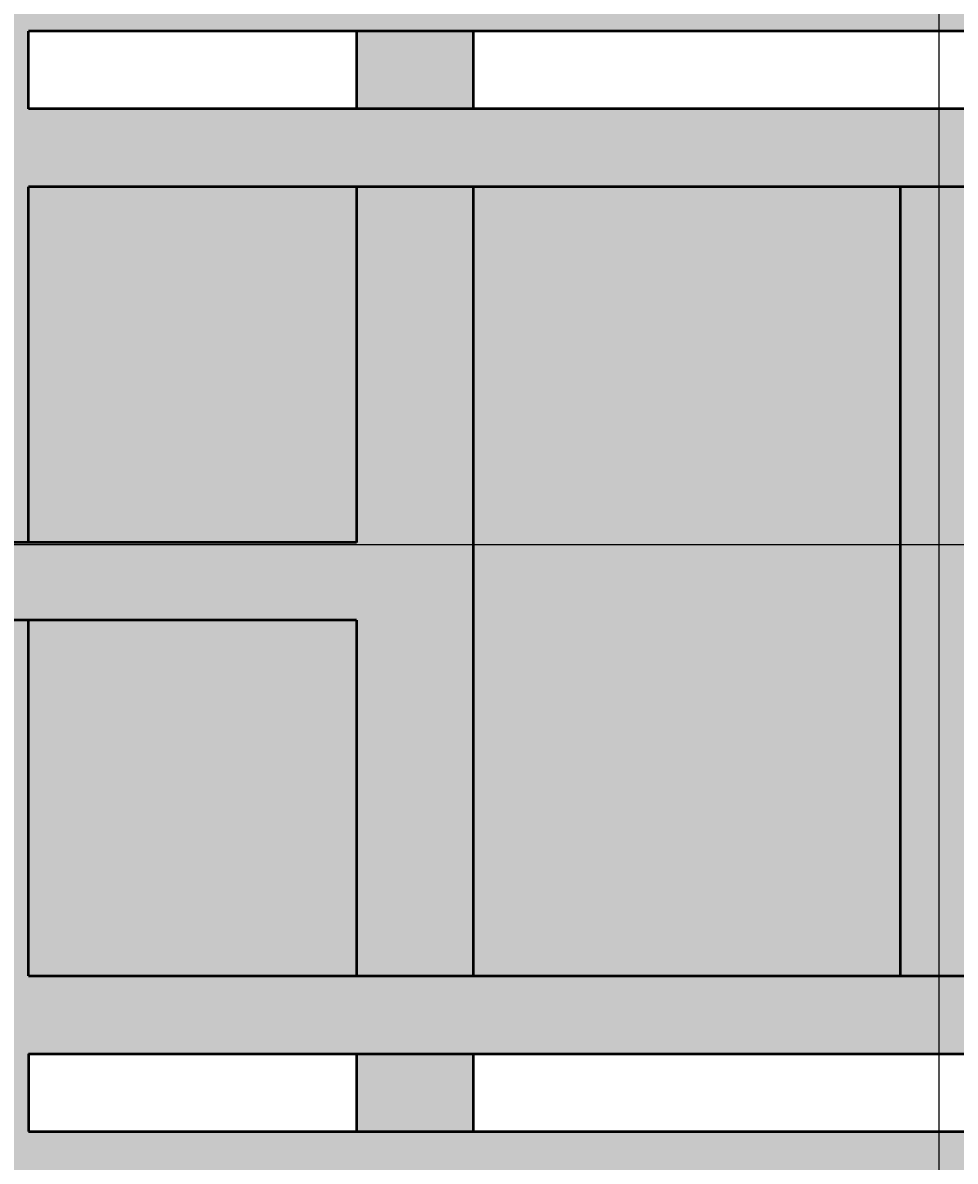
# Model space of a CAD drawing. Units: inches. Extents: x -12 to 334, y -10 to 186.
# Tile 17 of 77: x 64 to 88, y 65 to 94. Entities that reach past the tile are written whole.
import ezdxf

# ---------------------------------------------------------------- set-up
doc = ezdxf.new("R2010")
doc.units = ezdxf.units.IN
doc.header["$MEASUREMENT"] = 0
for name, color, linetype, lineweight in [('M-DIMS', 2, 'Continuous', 18), ('M-EQPM', 7, 'Continuous', 50), ('M-EQPM-PATT', 8, 'Continuous', 18)]:
    doc.layers.add(name, color=color, linetype=linetype, lineweight=lineweight)
doc.styles.get("Standard").update_dxf_attribs({"font": 'arial.ttf'})
doc.dimstyles.get("Standard").update_dxf_attribs({"dimtxt": 0.18, "dimasz": 0.18, "dimexe": 0.18, "dimexo": 0.0625, "dimgap": 0.09, "dimtad": 0, "dimtih": 1, "dimtoh": 1, "dimdec": 4, "dimzin": 0, "dimdsep": 46, "dimtxsty": 'Standard', "dimcen": 0.09, "dimadec": 0, "dimazin": 0, "dimtfac": 1, "dimtdec": 4, "dimtofl": 0, "dimtmove": 0, "dimatfit": 3, "dimfxl": 1, "dimtolj": 1, "dimtzin": 0, "dimarcsym": 0})

# ---------------------------------------------------------------- blocks, each defined once
blk = doc.blocks.new('*D1')
at = {"layer": 'Defpoints', "color": 0, "transparency": 16777216}
for p in [(281.426, 91.899), (3.376, 80.692), (281.426, 14.304)]:
    blk.add_point(p, dxfattribs=at)
at = {"layer": 'M-DIMS', "color": 0, "lineweight": -2, "transparency": 16777216}
for p, q in [((281.426, 91.836), (281.426, 14.124)), ((3.376, 80.629), (3.376, 14.124)), ((3.556, 14.304), (141.935, 14.304)), ((281.246, 14.304), (142.867, 14.304))]:
    blk.add_line(p, q, dxfattribs=at)
at = {"layer": 'M-DIMS', "color": 0, "transparency": 16777216}
for points in [[(3.556, 14.334), (3.556, 14.274), (3.376, 14.304)], [(281.246, 14.334), (281.246, 14.274), (281.426, 14.304)]]:
    blk.add_solid(points, dxfattribs=at)
at = {"layer": 'M-DIMS', "color": 0, "transparency": 16777216, "insert": (142.401, 14.304), "char_height": 0.18, "attachment_point": 5}
blk.add_mtext('\\A1;278.05', dxfattribs=at)
blk = doc.blocks.new('*D26')
at = {"layer": 'Defpoints', "color": 0, "transparency": 16777216}
for p in [(87.888, 169.385), (87.888, 56.321), (58.1, 33.675)]:
    blk.add_point(p, dxfattribs=at)
at = {"layer": 'M-DIMS', "color": 0, "lineweight": -2, "transparency": 16777216}
for p, q in [((58.1, 33.738), (58.1, 169.565)), ((87.888, 56.383), (87.888, 169.565)), ((58.28, 169.385), (72.599, 169.385)), ((87.708, 169.385), (73.389, 169.385))]:
    blk.add_line(p, q, dxfattribs=at)
at = {"layer": 'M-DIMS', "color": 0, "transparency": 16777216}
for points in [[(58.28, 169.415), (58.28, 169.355), (58.1, 169.385)], [(87.708, 169.415), (87.708, 169.355), (87.888, 169.385)]]:
    blk.add_solid(points, dxfattribs=at)
at = {"layer": 'M-DIMS', "color": 0, "transparency": 16777216, "insert": (72.994, 169.385), "char_height": 0.18, "attachment_point": 5}
blk.add_mtext('\\A1;29.79', dxfattribs=at)
blk = doc.blocks.new('*D35')
at = {"layer": 'Defpoints', "color": 0, "transparency": 16777216}
for p in [(216.428, 98.108), (-11.174, 61.105), (216.428, 61.105)]:
    blk.add_point(p, dxfattribs=at)
at = {"layer": 'M-DIMS', "color": 0, "lineweight": -2, "transparency": 16777216}
for p, q in [((216.365, 98.108), (-11.354, 98.108)), ((-11.174, 97.928), (-11.174, 79.788)), ((-11.174, 61.285), (-11.174, 79.424)), ((216.365, 61.105), (-11.354, 61.105))]:
    blk.add_line(p, q, dxfattribs=at)
at = {"layer": 'M-DIMS', "color": 0, "transparency": 16777216}
for points in [[(-11.204, 97.928), (-11.144, 97.928), (-11.174, 98.108)], [(-11.204, 61.285), (-11.144, 61.285), (-11.174, 61.105)]]:
    blk.add_solid(points, dxfattribs=at)
at = {"layer": 'M-DIMS', "color": 0, "transparency": 16777216, "insert": (-11.174, 79.606), "char_height": 0.18, "attachment_point": 5}
blk.add_mtext('\\A1;37', dxfattribs=at)
blk = doc.blocks.new('*D39')
at = {"layer": 'Defpoints', "color": 0, "transparency": 16777216}
for p in [(279.726, 80.692), (-11.174, 45.854), (269.381, 45.854)]:
    blk.add_point(p, dxfattribs=at)
at = {"layer": 'M-DIMS', "color": 0, "lineweight": -2, "transparency": 16777216}
for p, q in [((279.664, 80.692), (-11.354, 80.692)), ((-11.174, 80.512), (-11.174, 63.455)), ((-11.174, 46.034), (-11.174, 63.091)), ((269.318, 45.854), (-11.354, 45.854))]:
    blk.add_line(p, q, dxfattribs=at)
at = {"layer": 'M-DIMS', "color": 0, "transparency": 16777216}
for points in [[(-11.204, 80.512), (-11.144, 80.512), (-11.174, 80.692)], [(-11.204, 46.034), (-11.144, 46.034), (-11.174, 45.854)]]:
    blk.add_solid(points, dxfattribs=at)
at = {"layer": 'M-DIMS', "color": 0, "transparency": 16777216, "insert": (-11.174, 63.273), "char_height": 0.18, "attachment_point": 5}
blk.add_mtext('\\A1;34.84', dxfattribs=at)

msp = doc.modelspace()

# ---------------------------------------------------------------- hatches: boundary and pattern name
at = {"layer": 'M-EQPM-PATT'}
h = msp.add_hatch(color=256, dxfattribs=at)
h.set_gradient(color1=(99, 100, 102), color2=(99, 100, 102), tint=1)
h.paths.add_polyline_path([(4.3766, 80.754, -0.4132606), (23.5807, 99.8958), (37.1002, 99.8958), (37.1002, 127.7078), (32.1002, 127.7078), (32.1002, 125.2078), (36.1002, 125.2078), (36.1002, 100.8958), (23.5807, 100.8958, 1), (23.5807, 60.4872), (36.1002, 60.4872), (36.1002, 36.1752), (32.1002, 36.1752), (32.1002, 33.6752), (37.1002, 33.6752), (37.1002, 61.4872), (23.5807, 61.4872, -0.384914), (4.4744, 78.754), (72.9244, 78.754), (72.9244, 69.6117), (75.9244, 69.6117), (75.9244, 89.8963), (72.9244, 89.8963), (72.9244, 80.754)])
h.paths.add_polyline_path([(54.1002, 125.2078), (58.1002, 125.2078), (58.1002, 127.7078), (53.1002, 127.7078), (53.1002, 99.8958), (64.5, 99.8958), (64.5, 109.0583), (63.5, 109.0583), (63.5, 100.8958), (54.1002, 100.8958)], flags=17)
h.paths.add_polyline_path([(53.1002, 33.6752), (58.1002, 33.6752), (58.1002, 36.1752), (54.1002, 36.1752), (54.1002, 60.4872), (64.2068, 60.4872), (64.2068, 49.4497), (87.8879, 49.4497), (87.8879, 55.3205), (104.8919, 55.3205), (104.8919, 30.8541), (99.8919, 30.8541), (99.8919, 28.8541), (105.8919, 28.8541), (105.8919, 56.3205), (87.8879, 56.3205), (87.8879, 63.6117), (86.8879, 63.6117), (86.8879, 50.4497), (65.0061, 50.4497), (65.0061, 63.6117), (64.5, 63.6117), (64.5, 61.4872), (53.1002, 61.4872)])
h.paths.add_polyline_path([(121.8919, 28.8541), (121.8919, 30.8541), (116.8919, 30.8541), (116.8919, 45.8541), (209.6965, 45.8541), (209.9204, 46.8541), (115.8919, 46.8541), (115.8919, 28.8541)])
h.paths.add_polyline_path([(221.5761, 32.8541), (216.5761, 32.8541), (216.5761, 30.8541), (222.5761, 30.8541), (222.5761, 46.8541), (209.9204, 46.8541), (209.6965, 45.8541), (221.5761, 45.8541)])
h.paths.add_polyline_path([(233.5761, 45.8541), (249.8485, 45.8541), (249.3759, 46.8541), (232.5761, 46.8541), (232.5761, 30.8541), (238.5761, 30.8541), (238.5761, 32.8541), (233.5761, 32.8541)])
h = msp.add_hatch(color=256, dxfattribs=at)
h.set_gradient(color1=(205, 32, 39), color2=(205, 32, 39), tint=1)
h.paths.add_polyline_path([(64.5, 80.754), (64.5, 89.8963), (226.6083, 89.8963, -1), (226.6083, 69.6117), (64.5, 69.6117), (64.5, 78.754), (4.4744, 78.754, 0.384914), (23.5807, 61.4872), (37.1002, 61.4872), (37.1002, 33.6752), (53.1002, 33.6752), (53.1002, 61.4872), (64.5, 61.4872), (64.5, 63.6117), (226.6083, 63.6117, 1), (226.6083, 95.8963), (64.5, 95.8963), (64.5, 99.8958), (53.1002, 99.8958), (53.1002, 127.7078), (37.1002, 127.7078), (37.1002, 99.8958), (23.5807, 99.8958, 0.4132606), (4.3766, 80.754)])
h.paths.add_polyline_path([(64.5, 91.8963), (64.5, 93.8963), (226.6083, 93.8963, -1), (226.6083, 65.6117), (64.5, 65.6117), (64.5, 67.6117), (226.6083, 67.6117, 1), (226.6083, 91.8963)], flags=16)
h = msp.add_hatch(color=256, dxfattribs=at)
h.set_gradient(color1=(205, 32, 39), color2=(205, 32, 39), tint=1)
h.paths.add_polyline_path([(72.9244, 95.8963), (72.9244, 109.0583), (64.5, 109.0583), (64.5, 95.8963)])
h.paths.add_polyline_path([(72.9244, 80.754), (72.9244, 89.8963), (64.5, 89.8963), (64.5, 80.754)])
h.paths.add_polyline_path([(72.9244, 69.6117), (72.9244, 78.754), (64.5, 78.754), (64.5, 69.6117)])
h.paths.add_polyline_path([(72.9244, 50.4497), (72.9244, 63.6117), (65.0061, 63.6117), (65.0061, 50.4497)])
h = msp.add_hatch(color=256, dxfattribs=at)
h.set_gradient(color1=(99, 100, 102), color2=(99, 100, 102), tint=1)
h.paths.add_polyline_path([(72.9244, 95.8963), (75.9244, 95.8963), (75.9244, 109.0583), (72.9244, 109.0583)])
h.paths.add_polyline_path([(72.9244, 50.4497), (75.9244, 50.4497), (75.9244, 63.6117), (72.9244, 63.6117)])
h.paths.add_polyline_path([(75.9244, 91.8963), (75.9244, 93.8963), (72.9244, 93.8963), (72.9244, 91.8963)])
h.paths.add_polyline_path([(75.9244, 65.6117), (75.9244, 67.6117), (72.9244, 67.6117), (72.9244, 65.6117)])
h.paths.add_polyline_path([(129.093, 69.6117), (130.8573, 69.6117), (130.8573, 89.8963), (129.093, 89.8963)])
h.paths.add_polyline_path([(129.093, 98.1081), (129.093, 95.8963), (130.8573, 95.8963), (130.8573, 98.1081)])
h.paths.add_polyline_path([(130.8573, 61.1045), (130.8573, 63.6117), (129.093, 63.6117), (129.093, 61.1045)])
h.paths.add_polyline_path([(170.9079, 69.6117), (172.6722, 69.6117), (172.6722, 89.8963), (170.9079, 89.8963)])
h.paths.add_polyline_path([(172.6722, 95.8963), (172.6722, 98.1081), (170.9079, 98.1081), (170.9079, 95.8963)])
h.paths.add_polyline_path([(170.9079, 61.1045), (172.6722, 61.1045), (172.6722, 63.6117), (170.9079, 63.6117)])
h.paths.add_polyline_path([(218.1922, 63.6117), (216.4278, 63.6117), (216.4278, 61.1045), (218.1922, 61.1045)])
h.paths.add_polyline_path([(216.4278, 69.6117), (218.1922, 69.6117), (218.1922, 89.8963), (216.4278, 89.8963)])
h.paths.add_polyline_path([(216.4278, 95.8963), (218.1922, 95.8963), (218.1922, 98.1081), (216.4278, 98.1081)])
h = msp.add_hatch(color=256, dxfattribs=at)
h.set_gradient(color1=(94, 103, 175), color2=(94, 103, 175), tint=1)
h.paths.add_polyline_path([(129.093, 89.8963), (86.8879, 89.8963), (86.8879, 69.6117), (129.093, 69.6117)], flags=17)
h.paths.add_polyline_path([(170.9079, 89.8963), (130.8573, 89.8963), (130.8573, 69.6117), (170.9079, 69.6117)], flags=17)
h.paths.add_polyline_path([(216.4278, 89.8963), (172.6722, 89.8963), (172.6722, 69.6117), (216.4278, 69.6117)], flags=17)
h.paths.add_polyline_path([(245.9354, 82.6969), (247.9354, 82.6969), (247.9354, 46.8541), (268.3808, 46.8541, 0.0998398), (279.7263, 80.6915), (251.9801, 80.6915, 0.4142136), (231.7758, 100.8958), (84.7229, 100.8958), (84.7229, 109.0583), (83.7229, 109.0583), (83.7229, 95.8963), (129.093, 95.8963), (129.093, 98.1081), (130.8573, 98.1081), (130.8573, 95.8963), (170.9079, 95.8963), (170.9079, 98.1081), (172.6722, 98.1081), (172.6722, 95.8963), (216.4278, 95.8963), (216.4278, 98.1081), (218.1922, 98.1081), (218.1922, 95.8963), (226.6083, 95.8963, -1), (226.6083, 63.6117), (218.1922, 63.6117), (218.1922, 61.1045), (216.4278, 61.1045), (216.4278, 63.6117), (172.6722, 63.6117), (172.6722, 61.1045), (170.9079, 61.1045), (170.9079, 63.6117), (130.8573, 63.6117), (130.8573, 61.1045), (129.093, 61.1045), (129.093, 63.6117), (87.8879, 63.6117), (87.8879, 56.3205), (105.8919, 56.3205), (105.8919, 28.8541), (115.8919, 28.8541), (115.8919, 46.8541), (222.5761, 46.8541), (222.5761, 30.8541), (232.5761, 30.8541), (232.5761, 46.8541), (245.9354, 46.8541)])
h.paths.add_polyline_path([(86.8879, 89.8963), (75.9244, 89.8963), (75.9244, 69.6117), (86.8879, 69.6117)])
h.paths.add_polyline_path([(83.7229, 109.0583), (75.9244, 109.0583), (75.9244, 95.8963), (83.7229, 95.8963)])
h.paths.add_polyline_path([(226.6083, 89.8963), (218.1922, 89.8963), (218.1922, 69.6117), (226.6083, 69.6117, 1)], flags=17)

# ---------------------------------------------------------------- linework, layer by layer
at = {"layer": 'M-EQPM'}
for p, q in [((64.5, 91.8963), (64.5, 93.8963)), ((72.9244, 93.8963), (72.9244, 91.8963)), ((75.9244, 93.8963), (75.9244, 91.8963)), ((72.9244, 89.8963), (72.9244, 80.754)), ((75.9244, 89.8963), (75.9244, 69.6117)), ((72.9244, 80.754), (4.3766, 80.754)), ((72.9244, 78.754), (4.4744, 78.754)), ((72.9244, 78.754), (72.9244, 69.6117)), ((64.5, 67.6117), (64.5, 65.6117)), ((72.9244, 67.6117), (72.9244, 65.6117)), ((75.9244, 67.6117), (75.9244, 65.6117))]:
    msp.add_line(p, q, dxfattribs=at)
for points in [[(64.5, 65.6117), (226.6083, 65.6117, 1), (226.6083, 93.8963), (64.5, 93.8963)], [(64.5, 67.6117), (226.6083, 67.6117, 1), (226.6083, 91.8963), (64.5, 91.8963)], [(64.5, 69.6117), (226.6083, 69.6117, 1), (226.6083, 89.8963), (64.5, 89.8963)]]:
    msp.add_lwpolyline(points, format="xyb", dxfattribs=at)
for points in [[(64.5, 80.754), (64.5, 89.8963)], [(86.8879, 89.8963), (86.8879, 69.6117)], [(64.5, 69.6117), (64.5, 78.754)]]:
    msp.add_lwpolyline(points, dxfattribs=at)

# ---------------------------------------------------------------- dimensions: what is measured, and where the dimension line sits
at = {"layer": 'M-DIMS'}
for base, p1, p2, picture, middle in [((87.8879, 169.3845), (58.1002, 33.6752), (87.8879, 56.3205), '*D26', (72.9941, 169.3845)), ((281.4256, 14.3041), (3.3765, 80.6915), (281.4256, 91.8988), '*D1', (142.401, 14.3041))]:
    dim = msp.add_linear_dim(base=base, p1=p1, p2=p2, dimstyle='Standard', override={"dimdec": 2, "dimlfac": 1, "dimrnd": 0, "dimzin": 0, "dimdsep": 46, "dimlunit": 2}, dxfattribs=at)
    dim.commit()
    dim.dimension.update_dxf_attribs({"geometry": picture, "text_midpoint": middle})
for base, p1, p2, override, picture, middle in [((-11.1736, 61.1045), (216.4278, 98.1081), (216.4278, 61.1045), {"dimdec": 0, "dimlfac": 1, "dimrnd": 0, "dimzin": 0, "dimdsep": 46, "dimlunit": 2}, '*D35', (-11.1735, 79.6063)), ((-11.1736, 45.8541), (279.7263, 80.6915), (269.3808, 45.8541), {"dimdec": 2, "dimlfac": 1, "dimrnd": 0, "dimzin": 0, "dimdsep": 46, "dimlunit": 2}, '*D39', (-11.1735, 63.2728))]:
    dim = msp.add_linear_dim(base=base, p1=p1, p2=p2, angle=90, dimstyle='Standard', override=override, dxfattribs=at)
    dim.commit()
    dim.dimension.update_dxf_attribs({"geometry": picture, "text_midpoint": middle})

doc.saveas('drawing.dxf')
